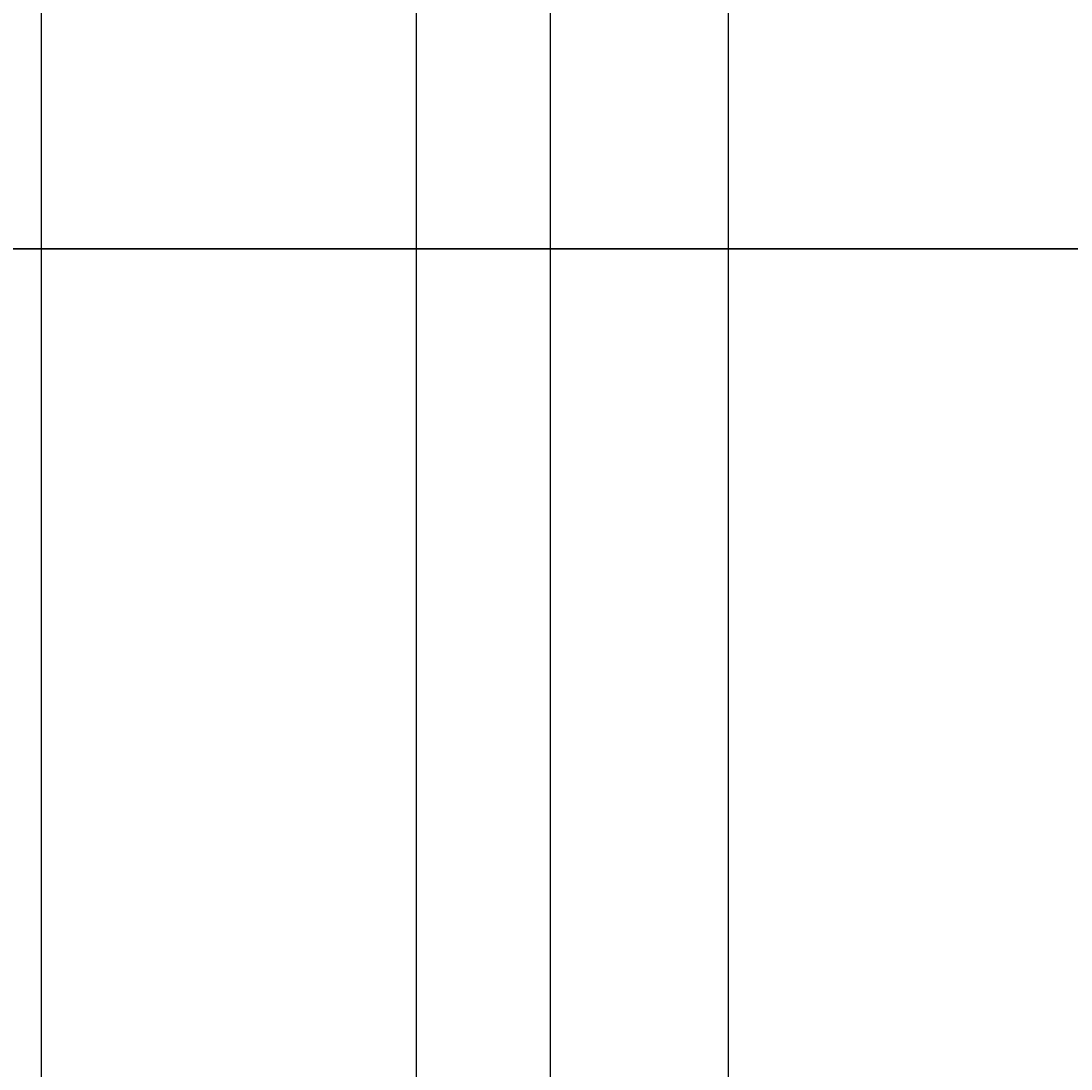
# Model space of a CAD drawing. Units: inches. Extents: x -6 to 289, y -8 to 323.
# Tile 78 of 107: x 126 to 150, y 229 to 252. Entities that reach past the tile are written whole.
import ezdxf

# ---------------------------------------------------------------- set-up
doc = ezdxf.new("R2010")
doc.units = ezdxf.units.IN
doc.header["$MEASUREMENT"] = 0
doc.layers.add('A-ANNO-DIMS', color=2, linetype='Continuous', lineweight=18)
doc.layers.add('A-ELEV', color=7, linetype='Continuous', lineweight=35)
doc.styles.get("Standard").update_dxf_attribs({"font": 'arial.ttf'})
doc.dimstyles.get("Standard").update_dxf_attribs({"dimtxt": 0.18, "dimasz": 0.18, "dimexe": 0.18, "dimexo": 0.0625, "dimgap": 0.09, "dimtad": 0, "dimtih": 1, "dimtoh": 1, "dimdec": 4, "dimzin": 0, "dimdsep": 46, "dimtxsty": 'Standard', "dimcen": 0.09, "dimadec": 0, "dimazin": 0, "dimtfac": 1, "dimtdec": 4, "dimtofl": 0, "dimtmove": 0, "dimatfit": 3, "dimfxl": 1, "dimtolj": 1, "dimtzin": 0, "dimarcsym": 0})

# ---------------------------------------------------------------- blocks, each defined once
blk = doc.blocks.new('*D10')
at = {"layer": 'A-ANNO-DIMS', "color": 0, "lineweight": -2, "transparency": 16777216}
for p, q in [((115.164, 307.351), (115.164, 322.969)), ((126.883, 226.717), (126.883, 322.969)), ((115.344, 322.789), (120.639, 322.789)), ((126.703, 322.789), (121.408, 322.789))]:
    blk.add_line(p, q, dxfattribs=at)
at = {"layer": 'A-ANNO-DIMS', "color": 0, "transparency": 16777216}
for points in [[(115.344, 322.819), (115.344, 322.759), (115.164, 322.789)], [(126.703, 322.819), (126.703, 322.759), (126.883, 322.789)]]:
    blk.add_solid(points, dxfattribs=at)
at = {"layer": 'Defpoints', "color": 0, "transparency": 16777216}
for p in [(126.883, 322.789), (115.164, 307.289), (126.883, 226.654)]:
    blk.add_point(p, dxfattribs=at)
at = {"layer": 'A-ANNO-DIMS', "color": 0, "transparency": 16777216, "insert": (121.024, 322.789), "char_height": 0.18, "attachment_point": 5}
blk.add_mtext('\\A1;11.72', dxfattribs=at)
blk = doc.blocks.new('*D11')
at = {"layer": 'A-ANNO-DIMS', "color": 0, "lineweight": -2, "transparency": 16777216}
for p, q in [((126.883, 226.717), (126.883, 322.969)), ((168.883, 226.717), (168.883, 322.969)), ((127.063, 322.789), (147.662, 322.789)), ((168.703, 322.789), (148.105, 322.789))]:
    blk.add_line(p, q, dxfattribs=at)
at = {"layer": 'A-ANNO-DIMS', "color": 0, "transparency": 16777216}
for points in [[(127.063, 322.819), (127.063, 322.759), (126.883, 322.789)], [(168.703, 322.819), (168.703, 322.759), (168.883, 322.789)]]:
    blk.add_solid(points, dxfattribs=at)
at = {"layer": 'Defpoints', "color": 0, "transparency": 16777216}
for p in [(168.883, 322.789), (126.883, 226.654), (168.883, 226.654)]:
    blk.add_point(p, dxfattribs=at)
at = {"layer": 'A-ANNO-DIMS', "color": 0, "transparency": 16777216, "insert": (147.883, 322.789), "char_height": 0.18, "attachment_point": 5}
blk.add_mtext('\\A1;42', dxfattribs=at)
blk = doc.blocks.new('*D26')
at = {"layer": 'A-ANNO-DIMS', "color": 0, "lineweight": -2, "transparency": 16777216}
for p, q in [((247.226, 247.289), (288.653, 247.289)), ((288.473, 247.109), (288.473, 237.153)), ((288.473, 226.834), (288.473, 236.789)), ((126.946, 226.654), (288.653, 226.654))]:
    blk.add_line(p, q, dxfattribs=at)
at = {"layer": 'A-ANNO-DIMS', "color": 0, "transparency": 16777216}
for points in [[(288.443, 247.109), (288.503, 247.109), (288.473, 247.289)], [(288.443, 226.834), (288.503, 226.834), (288.473, 226.654)]]:
    blk.add_solid(points, dxfattribs=at)
at = {"layer": 'Defpoints', "color": 0, "transparency": 16777216}
for p in [(247.164, 247.289), (288.473, 247.289), (126.883, 226.654)]:
    blk.add_point(p, dxfattribs=at)
at = {"layer": 'A-ANNO-DIMS', "color": 0, "transparency": 16777216, "insert": (288.473, 236.971), "char_height": 0.18, "attachment_point": 5}
blk.add_mtext('\\A1;20.635', dxfattribs=at)
blk = doc.blocks.new('*D27')
at = {"layer": 'A-ANNO-DIMS', "color": 0, "lineweight": -2, "transparency": 16777216}
for p, q in [((19.226, 307.289), (288.653, 307.289)), ((288.473, 307.109), (288.473, 277.471)), ((288.473, 247.469), (288.473, 277.107)), ((247.226, 247.289), (288.653, 247.289))]:
    blk.add_line(p, q, dxfattribs=at)
at = {"layer": 'A-ANNO-DIMS', "color": 0, "transparency": 16777216}
for points in [[(288.443, 307.109), (288.503, 307.109), (288.473, 307.289)], [(288.443, 247.469), (288.503, 247.469), (288.473, 247.289)]]:
    blk.add_solid(points, dxfattribs=at)
at = {"layer": 'Defpoints', "color": 0, "transparency": 16777216}
for p in [(19.164, 307.289), (288.473, 307.289), (247.164, 247.289)]:
    blk.add_point(p, dxfattribs=at)
at = {"layer": 'A-ANNO-DIMS', "color": 0, "transparency": 16777216, "insert": (288.473, 277.289), "char_height": 0.18, "attachment_point": 5}
blk.add_mtext('\\A1;60', dxfattribs=at)
blk = doc.blocks.new('*D73')
at = {"layer": 'A-ANNO-DIMS', "color": 0, "lineweight": -2, "transparency": 16777216}
for p, q in [((121.008, 51.148), (121.008, 322.969)), ((135.296, 51.148), (135.296, 322.969)), ((121.188, 322.789), (127.697, 322.789)), ((135.116, 322.789), (128.607, 322.789))]:
    blk.add_line(p, q, dxfattribs=at)
at = {"layer": 'A-ANNO-DIMS', "color": 0, "transparency": 16777216}
for points in [[(121.188, 322.819), (121.188, 322.759), (121.008, 322.789)], [(135.116, 322.819), (135.116, 322.759), (135.296, 322.789)]]:
    blk.add_solid(points, dxfattribs=at)
at = {"layer": 'Defpoints', "color": 0, "transparency": 16777216}
for p in [(135.296, 322.789), (121.008, 51.085), (135.296, 51.085)]:
    blk.add_point(p, dxfattribs=at)
at = {"layer": 'A-ANNO-DIMS', "color": 0, "transparency": 16777216, "insert": (128.152, 322.789), "char_height": 0.18, "attachment_point": 5}
blk.add_mtext('\\A1;14.288', dxfattribs=at)
blk = doc.blocks.new('*D74')
at = {"layer": 'A-ANNO-DIMS', "color": 0, "lineweight": -2, "transparency": 16777216}
for p, q in [((135.296, 51.148), (135.296, 322.969)), ((138.296, 51.148), (138.296, 322.969)), ((135.476, 322.789), (136.647, 322.789)), ((138.116, 322.789), (136.945, 322.789))]:
    blk.add_line(p, q, dxfattribs=at)
at = {"layer": 'A-ANNO-DIMS', "color": 0, "transparency": 16777216}
for points in [[(135.476, 322.819), (135.476, 322.759), (135.296, 322.789)], [(138.116, 322.819), (138.116, 322.759), (138.296, 322.789)]]:
    blk.add_solid(points, dxfattribs=at)
at = {"layer": 'Defpoints', "color": 0, "transparency": 16777216}
for p in [(138.296, 322.789), (135.296, 51.085), (138.296, 51.085)]:
    blk.add_point(p, dxfattribs=at)
at = {"layer": 'A-ANNO-DIMS', "color": 0, "transparency": 16777216, "insert": (136.796, 322.789), "char_height": 0.18, "attachment_point": 5}
blk.add_mtext('\\A1;3', dxfattribs=at)
blk = doc.blocks.new('*D75')
at = {"layer": 'A-ANNO-DIMS', "color": 0, "lineweight": -2, "transparency": 16777216}
for p, q in [((138.296, 51.148), (138.296, 322.969)), ((142.296, 51.148), (142.296, 322.969)), ((138.476, 322.789), (140.144, 322.789)), ((142.116, 322.789), (140.448, 322.789))]:
    blk.add_line(p, q, dxfattribs=at)
at = {"layer": 'A-ANNO-DIMS', "color": 0, "transparency": 16777216}
for points in [[(138.476, 322.819), (138.476, 322.759), (138.296, 322.789)], [(142.116, 322.819), (142.116, 322.759), (142.296, 322.789)]]:
    blk.add_solid(points, dxfattribs=at)
at = {"layer": 'Defpoints', "color": 0, "transparency": 16777216}
for p in [(142.296, 322.789), (138.296, 51.085), (142.296, 51.085)]:
    blk.add_point(p, dxfattribs=at)
at = {"layer": 'A-ANNO-DIMS', "color": 0, "transparency": 16777216, "insert": (140.296, 322.789), "char_height": 0.18, "attachment_point": 5}
blk.add_mtext('\\A1;4', dxfattribs=at)
blk = doc.blocks.new('*D76')
at = {"layer": 'A-ANNO-DIMS', "color": 0, "lineweight": -2, "transparency": 16777216}
for p, q in [((142.296, 51.148), (142.296, 322.969)), ((164.296, 51.148), (164.296, 322.969)), ((142.476, 322.789), (153.076, 322.789)), ((164.116, 322.789), (153.516, 322.789))]:
    blk.add_line(p, q, dxfattribs=at)
at = {"layer": 'A-ANNO-DIMS', "color": 0, "transparency": 16777216}
for points in [[(142.476, 322.819), (142.476, 322.759), (142.296, 322.789)], [(164.116, 322.819), (164.116, 322.759), (164.296, 322.789)]]:
    blk.add_solid(points, dxfattribs=at)
at = {"layer": 'Defpoints', "color": 0, "transparency": 16777216}
for p in [(164.296, 322.789), (142.296, 51.085), (164.296, 51.085)]:
    blk.add_point(p, dxfattribs=at)
at = {"layer": 'A-ANNO-DIMS', "color": 0, "transparency": 16777216, "insert": (153.296, 322.789), "char_height": 0.18, "attachment_point": 5}
blk.add_mtext('\\A1;22', dxfattribs=at)
blk = doc.blocks.new('*D94')
at = {"layer": 'A-ANNO-DIMS', "color": 0, "lineweight": -2, "transparency": 16777216}
for p, q in [((118.164, 159.411), (118.164, 322.969)), ((161.552, 159.411), (161.552, 322.969)), ((118.344, 322.789), (139.46, 322.789)), ((161.372, 322.789), (140.256, 322.789))]:
    blk.add_line(p, q, dxfattribs=at)
at = {"layer": 'A-ANNO-DIMS', "color": 0, "transparency": 16777216}
for points in [[(118.344, 322.819), (118.344, 322.759), (118.164, 322.789)], [(161.372, 322.819), (161.372, 322.759), (161.552, 322.789)]]:
    blk.add_solid(points, dxfattribs=at)
at = {"layer": 'Defpoints', "color": 0, "transparency": 16777216}
for p in [(161.552, 322.789), (118.164, 159.348), (161.552, 159.348)]:
    blk.add_point(p, dxfattribs=at)
at = {"layer": 'A-ANNO-DIMS', "color": 0, "transparency": 16777216, "insert": (139.858, 322.789), "char_height": 0.18, "attachment_point": 5}
blk.add_mtext('\\A1;43.39', dxfattribs=at)

msp = doc.modelspace()

# ---------------------------------------------------------------- linework, layer by layer
at = {"layer": 'A-ELEV'}
for p, q in [((247.1638, 247.2888), (115.1638, 247.2888)), ((115.1638, 247.2888), (247.1638, 247.2888))]:
    msp.add_line(p, q, dxfattribs=at)

# ---------------------------------------------------------------- dimensions: what is measured, and where the dimension line sits
at = {"layer": 'A-ANNO-DIMS'}
for base, p1, p2, override, picture, middle in [((126.8835, 322.7888), (115.1638, 307.2888), (126.8835, 226.654), {"dimdec": 2, "dimlfac": 1, "dimrnd": 0, "dimzin": 0, "dimdsep": 46, "dimlunit": 2}, '*D10', (121.0236, 322.7888)), ((161.5522, 322.7888), (118.1638, 159.3484), (161.5522, 159.3484), {"dimdec": 2, "dimlfac": 1, "dimrnd": 0, "dimzin": 0, "dimdsep": 46, "dimlunit": 2}, '*D94', (139.858, 322.7888)), ((135.296, 322.7888), (121.008, 51.0851), (135.296, 51.0851), {"dimdec": 3, "dimlfac": 1, "dimrnd": 0, "dimzin": 0, "dimdsep": 46, "dimlunit": 2}, '*D73', (128.152, 322.7888)), ((168.8835, 322.7888), (126.8835, 226.654), (168.8835, 226.654), {"dimdec": 0, "dimlfac": 1, "dimrnd": 0, "dimzin": 0, "dimdsep": 46, "dimlunit": 2}, '*D11', (147.8835, 322.7888)), ((138.296, 322.7888), (135.296, 51.0851), (138.296, 51.0851), {"dimdec": 0, "dimlfac": 1, "dimrnd": 0, "dimzin": 0, "dimdsep": 46, "dimlunit": 2}, '*D74', (136.796, 322.7888)), ((142.296, 322.7888), (138.296, 51.0851), (142.296, 51.0851), {"dimdec": 0, "dimlfac": 1, "dimrnd": 0, "dimzin": 0, "dimdsep": 46, "dimlunit": 2}, '*D75', (140.296, 322.7888)), ((164.296, 322.7888), (142.296, 51.0851), (164.296, 51.0851), {"dimdec": 0, "dimlfac": 1, "dimrnd": 0, "dimzin": 0, "dimdsep": 46, "dimlunit": 2}, '*D76', (153.296, 322.7888))]:
    dim = msp.add_linear_dim(base=base, p1=p1, p2=p2, dimstyle='Standard', override=override, dxfattribs=at)
    dim.commit()
    dim.dimension.update_dxf_attribs({"geometry": picture, "text_midpoint": middle})
for base, p1, p2, override, picture, middle in [((288.4733, 307.2888), (247.1638, 247.2888), (19.1638, 307.2888), {"dimdec": 0, "dimlfac": 1, "dimrnd": 0, "dimzin": 0, "dimdsep": 46, "dimlunit": 2}, '*D27', (288.4733, 277.2888)), ((288.4733, 247.2888), (126.8835, 226.654), (247.1638, 247.2888), {"dimdec": 3, "dimlfac": 1, "dimrnd": 0, "dimzin": 0, "dimdsep": 46, "dimlunit": 2}, '*D26', (288.4733, 236.9714))]:
    dim = msp.add_linear_dim(base=base, p1=p1, p2=p2, angle=90, dimstyle='Standard', override=override, dxfattribs=at)
    dim.commit()
    dim.dimension.update_dxf_attribs({"geometry": picture, "text_midpoint": middle})

doc.saveas('drawing.dxf')
